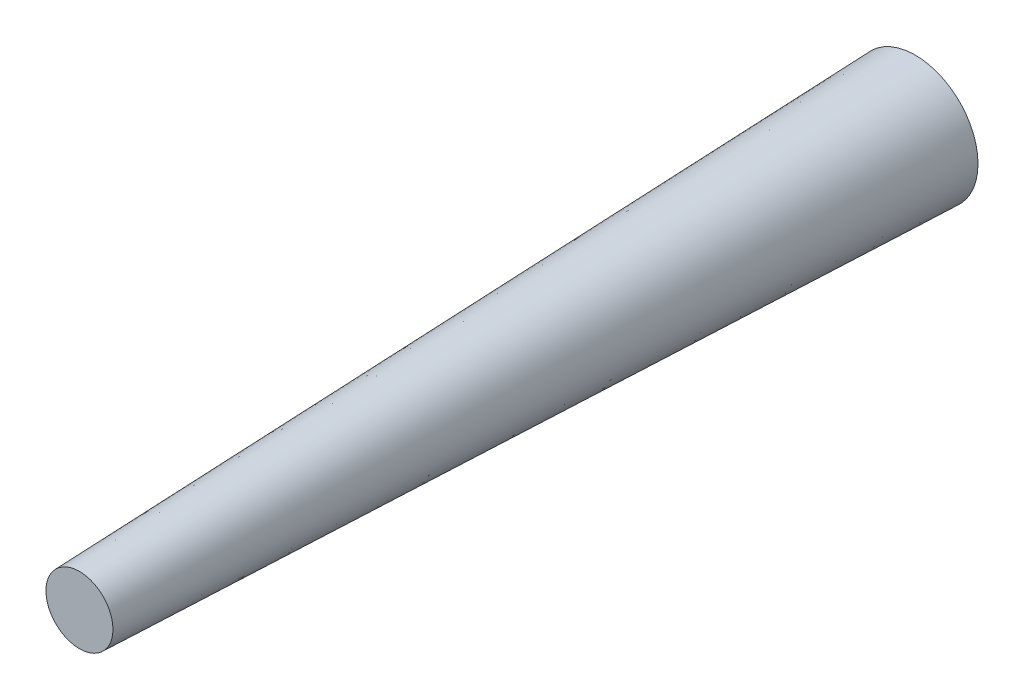
SolidWorks part; units mm, degrees
material "Plain Carbon Steel"
ref_plane "Front Plane" through (0, 0, 0) normal (0, 0, 1) x (1, 0, 0)
ref_plane "Top Plane" through (0, 0, 0) normal (0, 1, 0) x (1, 0, 0)
ref_plane "Right Plane" through (0, 0, 0) normal (1, 0, 0) x (0, 0, -1)
sketch "Pin Profile Ø6" plane through (0, 0, 0) normal (0, 0, 1) x (1, 0, 0)
  circle A0 centre (0, 0) radius 3
  dimension "D1" = 6
extrude "Taper Pin Body 40mm 2° Draft" add sketch "Pin Profile Ø6" along normal blind 40 draft 2
